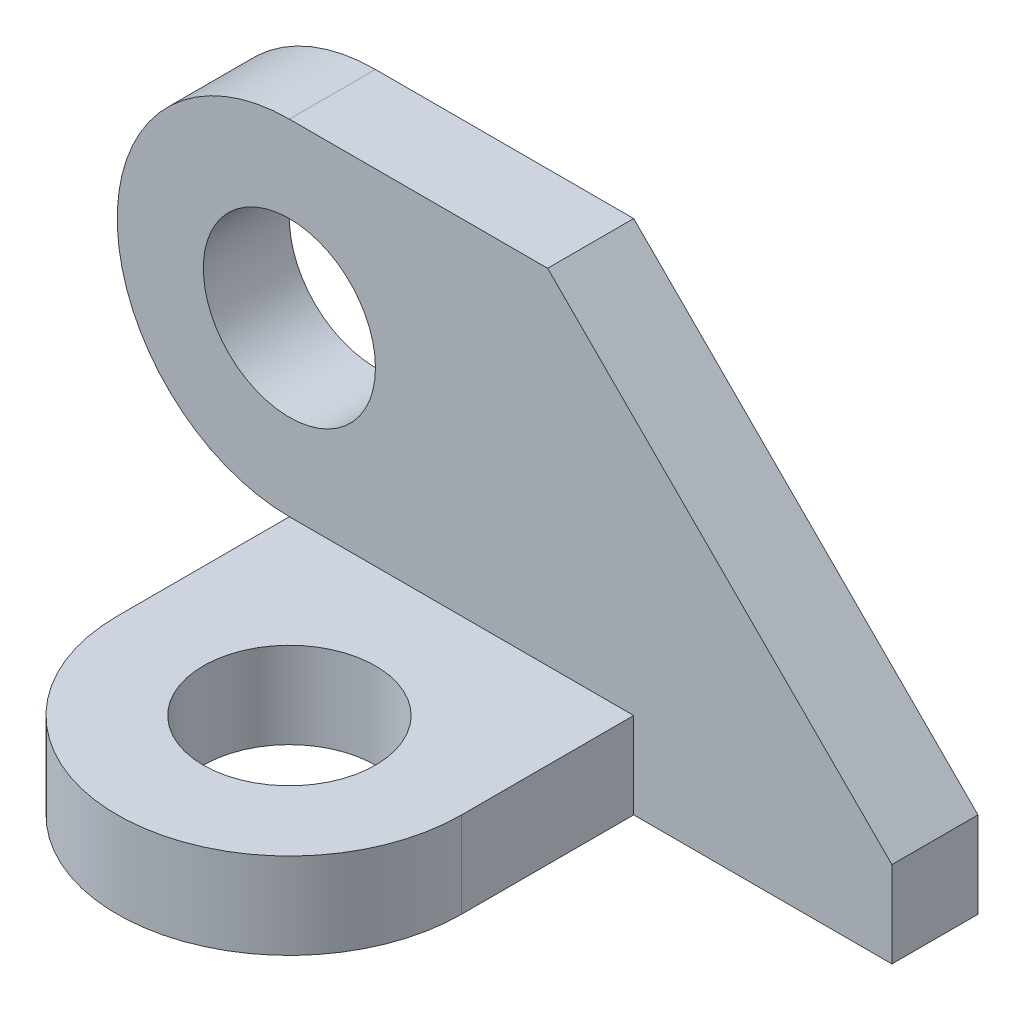
ISO-10303-21;
HEADER;
FILE_DESCRIPTION(('STEP AP214'),'2;1');
FILE_NAME('part.step','',(''),(''),'','','');
FILE_SCHEMA(('AUTOMOTIVE_DESIGN { 1 0 10303 214 1 1 1 1 }'));
ENDSEC;
DATA;
#1=APPLICATION_CONTEXT('core data for automotive mechanical design processes');
#2=APPLICATION_PROTOCOL_DEFINITION('international standard','automotive_design',2000,#1);
#3=PRODUCT_CONTEXT('',#1,'mechanical');
#4=PRODUCT('Part','Part','',(#3));
#5=PRODUCT_RELATED_PRODUCT_CATEGORY('part','',(#4));
#6=PRODUCT_DEFINITION_FORMATION('','',#4);
#7=PRODUCT_DEFINITION_CONTEXT('part definition',#1,'design');
#8=PRODUCT_DEFINITION('design','',#6,#7);
#9=PRODUCT_DEFINITION_SHAPE('','',#8);
#10=(LENGTH_UNIT() NAMED_UNIT(*) SI_UNIT(.MILLI.,.METRE.));
#11=(NAMED_UNIT(*) PLANE_ANGLE_UNIT() SI_UNIT($,.RADIAN.));
#12=(NAMED_UNIT(*) SI_UNIT($,.STERADIAN.) SOLID_ANGLE_UNIT());
#13=UNCERTAINTY_MEASURE_WITH_UNIT(LENGTH_MEASURE(1.E-05),#10,'distance_accuracy_value','');
#14=(GEOMETRIC_REPRESENTATION_CONTEXT(3) GLOBAL_UNCERTAINTY_ASSIGNED_CONTEXT((#13)) GLOBAL_UNIT_ASSIGNED_CONTEXT((#10,
#11,#12)) REPRESENTATION_CONTEXT('',''));
#15=CARTESIAN_POINT('',(0.,0.,0.));
#16=DIRECTION('',(0.,0.,1.));
#17=DIRECTION('',(1.,0.,0.));
#18=AXIS2_PLACEMENT_3D('',#15,#16,#17);
#19=CARTESIAN_POINT('',(0.,0.,5.));
#20=DIRECTION('',(1.,0.,0.));
#21=DIRECTION('',(0.,0.,-1.));
#22=AXIS2_PLACEMENT_3D('',#19,#20,#21);
#23=PLANE('',#22);
#24=DIRECTION('',(0.,-1.,0.));
#25=VECTOR('',#24,1.);
#26=CARTESIAN_POINT('',(0.,0.,-5.));
#27=LINE('',#26,#25);
#28=CARTESIAN_POINT('',(0.,10.,-5.));
#29=VERTEX_POINT('',#28);
#30=CARTESIAN_POINT('',(0.,0.,-5.));
#31=VERTEX_POINT('',#30);
#32=EDGE_CURVE('E129',#29,#31,#27,.T.);
#33=ORIENTED_EDGE('',*,*,#32,.T.);
#34=DIRECTION('',(0.,0.,-1.));
#35=VECTOR('',#34,1.);
#36=CARTESIAN_POINT('',(0.,0.,5.));
#37=LINE('',#36,#35);
#38=CARTESIAN_POINT('',(0.,0.,25.));
#39=VERTEX_POINT('',#38);
#40=EDGE_CURVE('E11',#39,#31,#37,.T.);
#41=ORIENTED_EDGE('',*,*,#40,.F.);
#42=DIRECTION('',(0.,-1.,0.));
#43=VECTOR('',#42,1.);
#44=CARTESIAN_POINT('',(0.,10.,25.));
#45=LINE('',#44,#43);
#46=CARTESIAN_POINT('',(0.,10.,25.));
#47=VERTEX_POINT('',#46);
#48=EDGE_CURVE('E165',#47,#39,#45,.T.);
#49=ORIENTED_EDGE('',*,*,#48,.F.);
#50=DIRECTION('',(0.,0.,-1.));
#51=VECTOR('',#50,1.);
#52=CARTESIAN_POINT('',(0.,10.,5.));
#53=LINE('',#52,#51);
#54=CARTESIAN_POINT('',(0.,10.,5.));
#55=VERTEX_POINT('',#54);
#56=EDGE_CURVE('E158',#47,#55,#53,.T.);
#57=ORIENTED_EDGE('',*,*,#56,.T.);
#58=DIRECTION('',(0.,0.,-1.));
#59=VECTOR('',#58,1.);
#60=CARTESIAN_POINT('',(0.,10.,5.));
#61=LINE('',#60,#59);
#62=EDGE_CURVE('E122',#55,#29,#61,.T.);
#63=ORIENTED_EDGE('',*,*,#62,.T.);
#64=EDGE_LOOP('',(#33,#41,#49,#57,#63));
#65=FACE_BOUND('',#64,.T.);
#66=ADVANCED_FACE('F39',(#65),#23,.F.);
#67=CARTESIAN_POINT('',(0.,0.,5.));
#68=DIRECTION('',(0.,1.,0.));
#69=DIRECTION('',(0.,0.,1.));
#70=AXIS2_PLACEMENT_3D('',#67,#68,#69);
#71=PLANE('',#70);
#72=CARTESIAN_POINT('',(20.,0.,25.));
#73=DIRECTION('',(0.,1.,0.));
#74=DIRECTION('',(0.,0.,1.));
#75=AXIS2_PLACEMENT_3D('',#72,#73,#74);
#76=CIRCLE('',#75,10.);
#77=CARTESIAN_POINT('',(20.,0.,35.));
#78=VERTEX_POINT('',#77);
#79=EDGE_CURVE('E182',#78,#78,#76,.T.);
#80=ORIENTED_EDGE('',*,*,#79,.T.);
#81=EDGE_LOOP('',(#80));
#82=FACE_BOUND('',#81,.T.);
#83=DIRECTION('',(1.,0.,0.));
#84=VECTOR('',#83,1.);
#85=CARTESIAN_POINT('',(0.,0.,-5.));
#86=LINE('',#85,#84);
#87=CARTESIAN_POINT('',(70.,0.,-5.));
#88=VERTEX_POINT('',#87);
#89=EDGE_CURVE('E131',#31,#88,#86,.T.);
#90=ORIENTED_EDGE('',*,*,#89,.T.);
#91=DIRECTION('',(0.,0.,-1.));
#92=VECTOR('',#91,1.);
#93=CARTESIAN_POINT('',(70.,0.,5.));
#94=LINE('',#93,#92);
#95=CARTESIAN_POINT('',(70.,0.,5.));
#96=VERTEX_POINT('',#95);
#97=EDGE_CURVE('E46',#96,#88,#94,.T.);
#98=ORIENTED_EDGE('',*,*,#97,.F.);
#99=DIRECTION('',(1.,0.,0.));
#100=VECTOR('',#99,1.);
#101=CARTESIAN_POINT('',(0.,0.,5.));
#102=LINE('',#101,#100);
#103=CARTESIAN_POINT('',(40.,0.,5.));
#104=VERTEX_POINT('',#103);
#105=EDGE_CURVE('E91',#104,#96,#102,.T.);
#106=ORIENTED_EDGE('',*,*,#105,.F.);
#107=DIRECTION('',(0.,0.,1.));
#108=VECTOR('',#107,1.);
#109=CARTESIAN_POINT('',(40.,0.,25.));
#110=LINE('',#109,#108);
#111=CARTESIAN_POINT('',(40.,0.,25.));
#112=VERTEX_POINT('',#111);
#113=EDGE_CURVE('E171',#104,#112,#110,.T.);
#114=ORIENTED_EDGE('',*,*,#113,.T.);
#115=CARTESIAN_POINT('',(20.,0.,25.));
#116=DIRECTION('',(0.,-1.,0.));
#117=DIRECTION('',(0.,0.,-1.));
#118=AXIS2_PLACEMENT_3D('',#115,#116,#117);
#119=CIRCLE('',#118,20.);
#120=EDGE_CURVE('E170',#112,#39,#119,.T.);
#121=ORIENTED_EDGE('',*,*,#120,.T.);
#122=ORIENTED_EDGE('',*,*,#40,.T.);
#123=EDGE_LOOP('',(#90,#98,#106,#114,#121,#122));
#124=FACE_BOUND('',#123,.T.);
#125=ADVANCED_FACE('F198',(#82,#124),#71,.F.);
#126=CARTESIAN_POINT('',(70.,0.,5.));
#127=DIRECTION('',(-1.,0.,0.));
#128=DIRECTION('',(0.,0.,1.));
#129=AXIS2_PLACEMENT_3D('',#126,#127,#128);
#130=PLANE('',#129);
#131=DIRECTION('',(0.,1.,0.));
#132=VECTOR('',#131,1.);
#133=CARTESIAN_POINT('',(70.,0.,-5.));
#134=LINE('',#133,#132);
#135=CARTESIAN_POINT('',(70.,10.,-5.));
#136=VERTEX_POINT('',#135);
#137=EDGE_CURVE('E133',#88,#136,#134,.T.);
#138=ORIENTED_EDGE('',*,*,#137,.T.);
#139=DIRECTION('',(0.,0.,-1.));
#140=VECTOR('',#139,1.);
#141=CARTESIAN_POINT('',(70.,10.,5.));
#142=LINE('',#141,#140);
#143=CARTESIAN_POINT('',(70.,10.,5.));
#144=VERTEX_POINT('',#143);
#145=EDGE_CURVE('E117',#144,#136,#142,.T.);
#146=ORIENTED_EDGE('',*,*,#145,.F.);
#147=DIRECTION('',(0.,1.,0.));
#148=VECTOR('',#147,1.);
#149=CARTESIAN_POINT('',(70.,0.,5.));
#150=LINE('',#149,#148);
#151=EDGE_CURVE('E107',#96,#144,#150,.T.);
#152=ORIENTED_EDGE('',*,*,#151,.F.);
#153=ORIENTED_EDGE('',*,*,#97,.T.);
#154=EDGE_LOOP('',(#138,#146,#152,#153));
#155=FACE_BOUND('',#154,.T.);
#156=ADVANCED_FACE('F144',(#155),#130,.F.);
#157=CARTESIAN_POINT('',(30.,50.,5.));
#158=DIRECTION('',(-0.707106781186547,-0.707106781186548,0.));
#159=DIRECTION('',(0.707106781186548,-0.707106781186547,0.));
#160=AXIS2_PLACEMENT_3D('',#157,#158,#159);
#161=PLANE('',#160);
#162=DIRECTION('',(-0.707106781186548,0.707106781186547,0.));
#163=VECTOR('',#162,1.);
#164=CARTESIAN_POINT('',(30.,50.,-5.));
#165=LINE('',#164,#163);
#166=CARTESIAN_POINT('',(30.,50.,-5.));
#167=VERTEX_POINT('',#166);
#168=EDGE_CURVE('E116',#136,#167,#165,.T.);
#169=ORIENTED_EDGE('',*,*,#168,.T.);
#170=DIRECTION('',(0.,0.,-1.));
#171=VECTOR('',#170,1.);
#172=CARTESIAN_POINT('',(30.,50.,5.));
#173=LINE('',#172,#171);
#174=CARTESIAN_POINT('',(30.,50.,5.));
#175=VERTEX_POINT('',#174);
#176=EDGE_CURVE('E111',#175,#167,#173,.T.);
#177=ORIENTED_EDGE('',*,*,#176,.F.);
#178=DIRECTION('',(-0.707106781186548,0.707106781186547,0.));
#179=VECTOR('',#178,1.);
#180=CARTESIAN_POINT('',(30.,50.,5.));
#181=LINE('',#180,#179);
#182=EDGE_CURVE('E101',#144,#175,#181,.T.);
#183=ORIENTED_EDGE('',*,*,#182,.F.);
#184=ORIENTED_EDGE('',*,*,#145,.T.);
#185=EDGE_LOOP('',(#169,#177,#183,#184));
#186=FACE_BOUND('',#185,.T.);
#187=ADVANCED_FACE('F113',(#186),#161,.F.);
#188=CARTESIAN_POINT('',(0.,50.,5.));
#189=DIRECTION('',(0.,-1.,0.));
#190=DIRECTION('',(0.,0.,-1.));
#191=AXIS2_PLACEMENT_3D('',#188,#189,#190);
#192=PLANE('',#191);
#193=DIRECTION('',(-1.,0.,0.));
#194=VECTOR('',#193,1.);
#195=CARTESIAN_POINT('',(0.,50.,-5.));
#196=LINE('',#195,#194);
#197=CARTESIAN_POINT('',(0.,50.,-5.));
#198=VERTEX_POINT('',#197);
#199=EDGE_CURVE('E140',#167,#198,#196,.T.);
#200=ORIENTED_EDGE('',*,*,#199,.T.);
#201=DIRECTION('',(0.,0.,-1.));
#202=VECTOR('',#201,1.);
#203=CARTESIAN_POINT('',(0.,50.,5.));
#204=LINE('',#203,#202);
#205=CARTESIAN_POINT('',(0.,50.,5.));
#206=VERTEX_POINT('',#205);
#207=EDGE_CURVE('E123',#206,#198,#204,.T.);
#208=ORIENTED_EDGE('',*,*,#207,.F.);
#209=DIRECTION('',(-1.,0.,0.));
#210=VECTOR('',#209,1.);
#211=CARTESIAN_POINT('',(0.,50.,5.));
#212=LINE('',#211,#210);
#213=EDGE_CURVE('E104',#175,#206,#212,.T.);
#214=ORIENTED_EDGE('',*,*,#213,.F.);
#215=ORIENTED_EDGE('',*,*,#176,.T.);
#216=EDGE_LOOP('',(#200,#208,#214,#215));
#217=FACE_BOUND('',#216,.T.);
#218=ADVANCED_FACE('F121',(#217),#192,.F.);
#219=CARTESIAN_POINT('',(0.,30.,5.));
#220=DIRECTION('',(0.,0.,-1.));
#221=DIRECTION('',(-1.,0.,0.));
#222=AXIS2_PLACEMENT_3D('',#219,#220,#221);
#223=CYLINDRICAL_SURFACE('',#222,20.);
#224=CARTESIAN_POINT('',(0.,30.,-5.));
#225=DIRECTION('',(0.,0.,1.));
#226=DIRECTION('',(1.,0.,0.));
#227=AXIS2_PLACEMENT_3D('',#224,#225,#226);
#228=CIRCLE('',#227,20.);
#229=EDGE_CURVE('E88',#198,#29,#228,.T.);
#230=ORIENTED_EDGE('',*,*,#229,.T.);
#231=ORIENTED_EDGE('',*,*,#62,.F.);
#232=CARTESIAN_POINT('',(0.,30.,5.));
#233=DIRECTION('',(0.,0.,1.));
#234=DIRECTION('',(1.,0.,0.));
#235=AXIS2_PLACEMENT_3D('',#232,#233,#234);
#236=CIRCLE('',#235,20.);
#237=EDGE_CURVE('E56',#206,#55,#236,.T.);
#238=ORIENTED_EDGE('',*,*,#237,.F.);
#239=ORIENTED_EDGE('',*,*,#207,.T.);
#240=EDGE_LOOP('',(#230,#231,#238,#239));
#241=FACE_BOUND('',#240,.T.);
#242=ADVANCED_FACE('F147',(#241),#223,.T.);
#243=CARTESIAN_POINT('',(0.,30.,5.));
#244=DIRECTION('',(0.,0.,1.));
#245=DIRECTION('',(1.,0.,0.));
#246=AXIS2_PLACEMENT_3D('',#243,#244,#245);
#247=PLANE('',#246);
#248=CARTESIAN_POINT('',(0.,30.,5.));
#249=DIRECTION('',(0.,0.,1.));
#250=DIRECTION('',(1.,0.,0.));
#251=AXIS2_PLACEMENT_3D('',#248,#249,#250);
#252=CIRCLE('',#251,10.);
#253=CARTESIAN_POINT('',(10.,30.,5.));
#254=VERTEX_POINT('',#253);
#255=EDGE_CURVE('E240',#254,#254,#252,.T.);
#256=ORIENTED_EDGE('',*,*,#255,.F.);
#257=EDGE_LOOP('',(#256));
#258=FACE_BOUND('',#257,.T.);
#259=DIRECTION('',(0.,-1.,0.));
#260=VECTOR('',#259,1.);
#261=CARTESIAN_POINT('',(40.,10.,5.));
#262=LINE('',#261,#260);
#263=CARTESIAN_POINT('',(40.,10.,5.));
#264=VERTEX_POINT('',#263);
#265=EDGE_CURVE('E179',#264,#104,#262,.T.);
#266=ORIENTED_EDGE('',*,*,#265,.T.);
#267=ORIENTED_EDGE('',*,*,#105,.T.);
#268=ORIENTED_EDGE('',*,*,#151,.T.);
#269=ORIENTED_EDGE('',*,*,#182,.T.);
#270=ORIENTED_EDGE('',*,*,#213,.T.);
#271=ORIENTED_EDGE('',*,*,#237,.T.);
#272=DIRECTION('',(1.,0.,0.));
#273=VECTOR('',#272,1.);
#274=CARTESIAN_POINT('',(0.,10.,5.));
#275=LINE('',#274,#273);
#276=EDGE_CURVE('E52',#55,#264,#275,.T.);
#277=ORIENTED_EDGE('',*,*,#276,.T.);
#278=EDGE_LOOP('',(#266,#267,#268,#269,#270,#271,#277));
#279=FACE_BOUND('',#278,.T.);
#280=ADVANCED_FACE('F103',(#258,#279),#247,.T.);
#281=CARTESIAN_POINT('',(0.,30.,-5.));
#282=DIRECTION('',(0.,0.,1.));
#283=DIRECTION('',(1.,0.,0.));
#284=AXIS2_PLACEMENT_3D('',#281,#282,#283);
#285=PLANE('',#284);
#286=CARTESIAN_POINT('',(0.,30.,-5.));
#287=DIRECTION('',(0.,0.,1.));
#288=DIRECTION('',(1.,0.,0.));
#289=AXIS2_PLACEMENT_3D('',#286,#287,#288);
#290=CIRCLE('',#289,10.);
#291=CARTESIAN_POINT('',(10.,30.,-5.));
#292=VERTEX_POINT('',#291);
#293=EDGE_CURVE('E239',#292,#292,#290,.T.);
#294=ORIENTED_EDGE('',*,*,#293,.T.);
#295=EDGE_LOOP('',(#294));
#296=FACE_BOUND('',#295,.T.);
#297=ORIENTED_EDGE('',*,*,#32,.F.);
#298=ORIENTED_EDGE('',*,*,#229,.F.);
#299=ORIENTED_EDGE('',*,*,#199,.F.);
#300=ORIENTED_EDGE('',*,*,#168,.F.);
#301=ORIENTED_EDGE('',*,*,#137,.F.);
#302=ORIENTED_EDGE('',*,*,#89,.F.);
#303=EDGE_LOOP('',(#297,#298,#299,#300,#301,#302));
#304=FACE_BOUND('',#303,.T.);
#305=ADVANCED_FACE('F149',(#296,#304),#285,.F.);
#306=CARTESIAN_POINT('',(20.,10.,25.));
#307=DIRECTION('',(0.,-1.,0.));
#308=DIRECTION('',(0.,0.,-1.));
#309=AXIS2_PLACEMENT_3D('',#306,#307,#308);
#310=CYLINDRICAL_SURFACE('',#309,20.);
#311=ORIENTED_EDGE('',*,*,#120,.F.);
#312=DIRECTION('',(0.,-1.,0.));
#313=VECTOR('',#312,1.);
#314=CARTESIAN_POINT('',(40.,10.,25.));
#315=LINE('',#314,#313);
#316=CARTESIAN_POINT('',(40.,10.,25.));
#317=VERTEX_POINT('',#316);
#318=EDGE_CURVE('E184',#317,#112,#315,.T.);
#319=ORIENTED_EDGE('',*,*,#318,.F.);
#320=CARTESIAN_POINT('',(20.,10.,25.));
#321=DIRECTION('',(0.,-1.,0.));
#322=DIRECTION('',(0.,0.,-1.));
#323=AXIS2_PLACEMENT_3D('',#320,#321,#322);
#324=CIRCLE('',#323,20.);
#325=EDGE_CURVE('E166',#317,#47,#324,.T.);
#326=ORIENTED_EDGE('',*,*,#325,.T.);
#327=ORIENTED_EDGE('',*,*,#48,.T.);
#328=EDGE_LOOP('',(#311,#319,#326,#327));
#329=FACE_BOUND('',#328,.T.);
#330=ADVANCED_FACE('F203',(#329),#310,.T.);
#331=CARTESIAN_POINT('',(40.,10.,25.));
#332=DIRECTION('',(1.,0.,0.));
#333=DIRECTION('',(0.,0.,-1.));
#334=AXIS2_PLACEMENT_3D('',#331,#332,#333);
#335=PLANE('',#334);
#336=ORIENTED_EDGE('',*,*,#113,.F.);
#337=ORIENTED_EDGE('',*,*,#265,.F.);
#338=DIRECTION('',(0.,0.,1.));
#339=VECTOR('',#338,1.);
#340=CARTESIAN_POINT('',(40.,10.,25.));
#341=LINE('',#340,#339);
#342=EDGE_CURVE('E161',#264,#317,#341,.T.);
#343=ORIENTED_EDGE('',*,*,#342,.T.);
#344=ORIENTED_EDGE('',*,*,#318,.T.);
#345=EDGE_LOOP('',(#336,#337,#343,#344));
#346=FACE_BOUND('',#345,.T.);
#347=ADVANCED_FACE('F191',(#346),#335,.T.);
#348=CARTESIAN_POINT('',(20.,10.,25.));
#349=DIRECTION('',(0.,-1.,0.));
#350=DIRECTION('',(0.,0.,-1.));
#351=AXIS2_PLACEMENT_3D('',#348,#349,#350);
#352=PLANE('',#351);
#353=CARTESIAN_POINT('',(20.,10.,25.));
#354=DIRECTION('',(0.,1.,0.));
#355=DIRECTION('',(0.,0.,1.));
#356=AXIS2_PLACEMENT_3D('',#353,#354,#355);
#357=CIRCLE('',#356,10.);
#358=CARTESIAN_POINT('',(20.,10.,35.));
#359=VERTEX_POINT('',#358);
#360=EDGE_CURVE('E172',#359,#359,#357,.T.);
#361=ORIENTED_EDGE('',*,*,#360,.F.);
#362=EDGE_LOOP('',(#361));
#363=FACE_BOUND('',#362,.T.);
#364=ORIENTED_EDGE('',*,*,#276,.F.);
#365=ORIENTED_EDGE('',*,*,#56,.F.);
#366=ORIENTED_EDGE('',*,*,#325,.F.);
#367=ORIENTED_EDGE('',*,*,#342,.F.);
#368=EDGE_LOOP('',(#364,#365,#366,#367));
#369=FACE_BOUND('',#368,.T.);
#370=ADVANCED_FACE('F156',(#363,#369),#352,.F.);
#371=CARTESIAN_POINT('',(20.,0.,25.));
#372=DIRECTION('',(0.,1.,0.));
#373=DIRECTION('',(0.,0.,1.));
#374=AXIS2_PLACEMENT_3D('',#371,#372,#373);
#375=CYLINDRICAL_SURFACE('',#374,10.);
#376=ORIENTED_EDGE('',*,*,#79,.F.);
#377=EDGE_LOOP('',(#376));
#378=FACE_BOUND('',#377,.T.);
#379=ORIENTED_EDGE('',*,*,#360,.T.);
#380=EDGE_LOOP('',(#379));
#381=FACE_BOUND('',#380,.T.);
#382=ADVANCED_FACE('F250',(#378,#381),#375,.F.);
#383=CARTESIAN_POINT('',(0.,30.,-5.));
#384=DIRECTION('',(0.,0.,1.));
#385=DIRECTION('',(1.,0.,0.));
#386=AXIS2_PLACEMENT_3D('',#383,#384,#385);
#387=CYLINDRICAL_SURFACE('',#386,10.);
#388=ORIENTED_EDGE('',*,*,#293,.F.);
#389=EDGE_LOOP('',(#388));
#390=FACE_BOUND('',#389,.T.);
#391=ORIENTED_EDGE('',*,*,#255,.T.);
#392=EDGE_LOOP('',(#391));
#393=FACE_BOUND('',#392,.T.);
#394=ADVANCED_FACE('F253',(#390,#393),#387,.F.);
#395=CLOSED_SHELL('',(#66,#125,#156,#187,#218,#242,#280,#305,#330,#347,#370,#382,#394));
#396=MANIFOLD_SOLID_BREP('B2',#395);
#397=ADVANCED_BREP_SHAPE_REPRESENTATION('',(#18,#396),#14);
#398=SHAPE_DEFINITION_REPRESENTATION(#9,#397);
ENDSEC;
END-ISO-10303-21;
